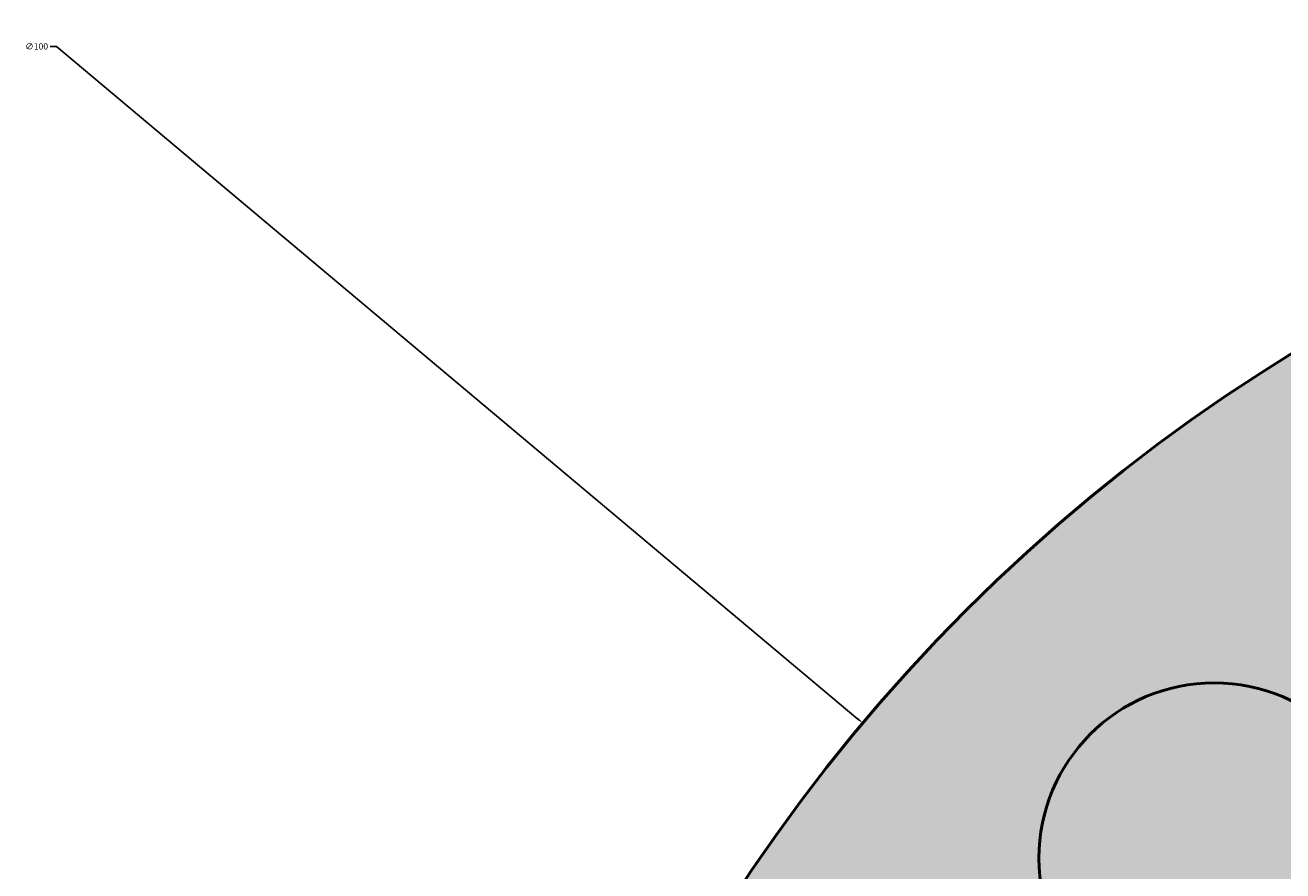
# Model space of a CAD drawing. Units: inches. Extents: x 139261 to 139415, y 52839 to 52963.
# Tile 6 of 20: x 139278 to 139314, y 52928 to 52952. Entities that reach past the tile are written whole.
import ezdxf

# ---------------------------------------------------------------- set-up
doc = ezdxf.new("R2010")
doc.units = ezdxf.units.IN
doc.header["$MEASUREMENT"] = 0
for name, color, linetype, lineweight in [('M-DIMS', 2, 'Continuous', 25), ('M-HATC', 8, 'Continuous', 18), ('M-OUTL', 7, 'Continuous', 50)]:
    doc.layers.add(name, color=color, linetype=linetype, lineweight=lineweight)
doc.styles.get("Standard").update_dxf_attribs({"font": 'arial.ttf'})
doc.dimstyles.get("Standard").update_dxf_attribs({"dimtxt": 0.18, "dimasz": 0.18, "dimexe": 0.18, "dimexo": 0.0625, "dimgap": 0.09, "dimtad": 0, "dimtih": 1, "dimtoh": 1, "dimdec": 4, "dimzin": 0, "dimdsep": 46, "dimtxsty": 'Standard', "dimcen": 0.09, "dimadec": 0, "dimazin": 0, "dimtfac": 1, "dimtdec": 4, "dimtofl": 0, "dimtmove": 0, "dimatfit": 3, "dimfxl": 1, "dimtolj": 1, "dimtzin": 0, "dimarcsym": 0})

# ---------------------------------------------------------------- blocks, each defined once
blk = doc.blocks.new('*U1')
blk.add_circle((0, 0), 5)
blk = doc.blocks.new('*U2')
at = {"layer": 'M-OUTL', "color": 0, "linetype": 'ByBlock', "lineweight": -2, "transparency": 16777216, "rotation": 45.00000000000001}
blk.add_blockref('*U1', (139312.073, 52928.502), dxfattribs=at)
blk = doc.blocks.new('*D4')
at = {"layer": 'Defpoints', "color": 0, "transparency": 16777216}
for p in [(139373.053, 52923.26), (139307.661, 52877.175)]:
    blk.add_point(p, dxfattribs=at)
at = {"layer": 'M-DIMS', "color": 0, "lineweight": -2, "transparency": 16777216}
for p, q in [((139414.011, 52952.126), (139373.2, 52923.364)), ((139414.191, 52952.126), (139414.011, 52952.126)), ((139340.267, 52900.217), (139340.447, 52900.217)), ((139340.357, 52900.127), (139340.357, 52900.307))]:
    blk.add_line(p, q, dxfattribs=at)
blk.add_arc((139340.357, 52900.217), 40, 34.9168, 52.0771, dxfattribs=at)
at = {"layer": 'M-DIMS', "color": 0, "transparency": 16777216}
blk.add_solid([(139373.183, 52923.388), (139373.217, 52923.339), (139373.053, 52923.26)], dxfattribs=at)
at = {"layer": 'M-DIMS', "color": 0, "transparency": 16777216, "insert": (139414.822, 52952.126), "char_height": 0.18, "attachment_point": 5}
blk.add_mtext('\\A1;∅80.0000', dxfattribs=at)
blk = doc.blocks.new('*D9')
at = {"layer": 'Defpoints', "color": 0, "transparency": 16777216}
for p in [(139302.054, 52932.357), (139378.659, 52868.078)]:
    blk.add_point(p, dxfattribs=at)
at = {"layer": 'M-DIMS', "color": 0, "lineweight": -2, "transparency": 16777216}
for p, q in [((139278.893, 52951.64), (139279.073, 52951.64)), ((139279.073, 52951.64), (139301.916, 52932.472)), ((139340.267, 52900.217), (139340.447, 52900.217)), ((139340.357, 52900.127), (139340.357, 52900.307))]:
    blk.add_line(p, q, dxfattribs=at)
at = {"layer": 'M-DIMS', "color": 0, "transparency": 16777216}
blk.add_solid([(139301.936, 52932.495), (139301.897, 52932.449), (139302.054, 52932.357)], dxfattribs=at)
at = {"layer": 'M-DIMS', "color": 0, "transparency": 16777216, "insert": (139278.506, 52951.64), "char_height": 0.18, "attachment_point": 5}
blk.add_mtext('\\A1;∅100', dxfattribs=at)

msp = doc.modelspace()

# ---------------------------------------------------------------- hatches: boundary and pattern name
at = {"layer": 'M-HATC'}
h = msp.add_hatch(color=256, dxfattribs=at)
h.dxf.hatch_style = 1
h.paths.add_polyline_path([(139290.35689, 52900.21749, 1), (139390.35689, 52900.21749, 1)])
h.paths.add_polyline_path([(139335.36666, 52939.90499, -0.01563646), (139335.35689, 52940.21749, -1), (139345.35689, 52940.21749, -0.01563646), (139345.34711, 52939.90499, -0.13461315), (139364.89157, 52931.80941, -0.691035), (139373.64116, 52928.50176, -0.21521822), (139371.94881, 52924.75216, -0.13461315), (139380.04439, 52905.20771, -0.43265224), (139385.35689, 52900.21749, -0.43265224), (139380.04439, 52895.22726, -0.13461315), (139371.94881, 52875.68281, -0.21521822), (139373.64116, 52871.93321, -0.691035), (139364.89157, 52868.62556, -0.13461315), (139345.34711, 52860.52999, -0.01563646), (139345.35689, 52860.21749, -1), (139335.35689, 52860.21749, -0.01563646), (139335.36666, 52860.52999, -0.13461315), (139315.82221, 52868.62556, -0.691035), (139307.07262, 52871.93321, -0.21521822), (139308.76496, 52875.68281, -0.13461315), (139300.66939, 52895.22726, -0.43265224), (139295.35689, 52900.21749, -0.43265224), (139300.66939, 52905.20771, -0.13461315), (139308.76496, 52924.75216, -0.21521822), (139307.07262, 52928.50176, -0.691035), (139315.82221, 52931.80941, -0.13461315)], flags=16)
h.paths.add_polyline_path([(139365.35689, 52900.21749, -1), (139315.35689, 52900.21749, -1)], flags=0)
h.paths.add_polyline_path([(139323.71474, 52911.30978), (139356.99903, 52911.30978, -0.3027197), (139356.99903, 52889.12519), (139323.71474, 52889.12519, -0.3027197)], flags=0)
h.paths.add_polyline_path([(139364.89157, 52931.80941, 0.13461315), (139345.34711, 52939.90499, -0.93933644), (139335.36666, 52939.90499, 0.13461315), (139315.82221, 52931.80941, -0.18270763), (139317.07262, 52928.50176, -0.64579494), (139308.76496, 52924.75216, 0.13461315), (139300.66939, 52905.20771, -0.39601219), (139305.35689, 52900.21749, -0.39601219), (139300.66939, 52895.22726, 0.13461315), (139308.76496, 52875.68281, -0.64579494), (139317.07262, 52871.93321, -0.18270763), (139315.82221, 52868.62556, 0.13461315), (139335.36666, 52860.52999, -0.93933644), (139345.34711, 52860.52999, 0.13461315), (139364.89157, 52868.62556, -0.18270763), (139363.64116, 52871.93321, -0.64579494), (139371.94881, 52875.68281, 0.13461315), (139380.04439, 52895.22726, -0.39601219), (139375.35689, 52900.21749, -0.39601219), (139380.04439, 52905.20771, 0.13461315), (139371.94881, 52924.75216, -0.64579494), (139363.64116, 52928.50176, -0.18270763)], flags=0)
h = msp.add_hatch(color=256, dxfattribs=at)
h.dxf.hatch_style = 1
h.set_gradient(color1=(205, 105, 40), tint=1)
h.paths.add_polyline_path([(139335.35689, 52940.21749, 1), (139345.35689, 52940.21749, 1)])
h.paths.add_polyline_path([(139307.07262, 52928.50176, 1), (139317.07262, 52928.50176, 1)])
h.paths.add_polyline_path([(139295.35689, 52900.21749, 1), (139305.35689, 52900.21749, 1)])
h.paths.add_polyline_path([(139307.07262, 52871.93321, 1), (139317.07262, 52871.93321, 1)])
h.paths.add_polyline_path([(139345.35689, 52860.21749, 1), (139335.35689, 52860.21749, 1)])
h.paths.add_polyline_path([(139363.64116, 52871.93321, 1), (139373.64116, 52871.93321, 1)])
h.paths.add_polyline_path([(139375.35689, 52900.21749, 1), (139385.35689, 52900.21749, 1)])
h.paths.add_polyline_path([(139363.64116, 52928.50176, 1), (139373.64116, 52928.50176, 1)])
h = msp.add_hatch(color=256, dxfattribs=at)
h.dxf.hatch_style = 1
h.paths.add_polyline_path([(139345.34711, 52939.90499, -0.93933644), (139335.36666, 52939.90499, 0.13461315), (139315.82221, 52931.80941, -0.18270763), (139317.07262, 52928.50176, -0.64579494), (139308.76496, 52924.75216, 0.13461315), (139300.66939, 52905.20771, -0.39601219), (139305.35689, 52900.21749, -0.39601219), (139300.66939, 52895.22726, 0.13461315), (139308.76496, 52875.68281, -0.64579494), (139317.07262, 52871.93321, -0.18270763), (139315.82221, 52868.62556, 0.13461315), (139335.36666, 52860.52999, -0.93933644), (139345.34711, 52860.52999, 0.13461315), (139364.89157, 52868.62556, -0.18270763), (139363.64116, 52871.93321, -0.64579494), (139371.94881, 52875.68281, 0.13461315), (139380.04439, 52895.22726, -0.39601219), (139375.35689, 52900.21749, -0.39601219), (139380.04439, 52905.20771, 0.13461315), (139371.94881, 52924.75216, -0.64579494), (139363.64116, 52928.50176, -0.18270763), (139364.89157, 52931.80941, 0.13461315)])
h.paths.add_polyline_path([(139365.35689, 52900.21749, -1), (139315.35689, 52900.21749, -1)], flags=16)
h.paths.add_polyline_path([(139356.99903, 52911.30978, -0.3027197), (139356.99903, 52889.12519), (139323.71474, 52889.12519, -0.3027197), (139323.71474, 52911.30978)], flags=0)

# ---------------------------------------------------------------- linework, layer by layer
at = {"layer": 'M-OUTL'}
msp.add_circle((139340.35689, 52900.21749), 50, dxfattribs=at)

# ---------------------------------------------------------------- block references
msp.add_blockref('*U2', (0, 0), dxfattribs=at)

# ---------------------------------------------------------------- dimensions: what is measured, and where the dimension line sits
at = {"layer": 'M-DIMS'}
for p1, p2, override, picture, middle in [((139307.66087, 52877.17469), (139373.0529, 52923.26028), {"dimclrd": 0, "dimclre": 0, "dimclrt": 0}, '*D4', (139414.82217, 52952.12585)), ((139378.65939, 52868.07845), (139302.05438, 52932.35652), {"dimdec": 0, "dimlfac": 1, "dimrnd": 0, "dimzin": 0, "dimdsep": 46, "dimlunit": 2}, '*D9', (139278.50641, 52951.63995))]:
    dim = msp.add_diameter_dim_2p(p1=p1, p2=p2, dimstyle='Standard', override=override, dxfattribs=at)
    dim.commit()
    dim.dimension.update_dxf_attribs({"geometry": picture, "text_midpoint": middle, "dimtype": 163})

doc.saveas('drawing.dxf')
